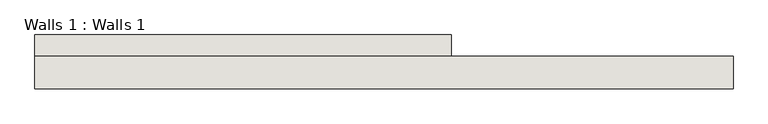
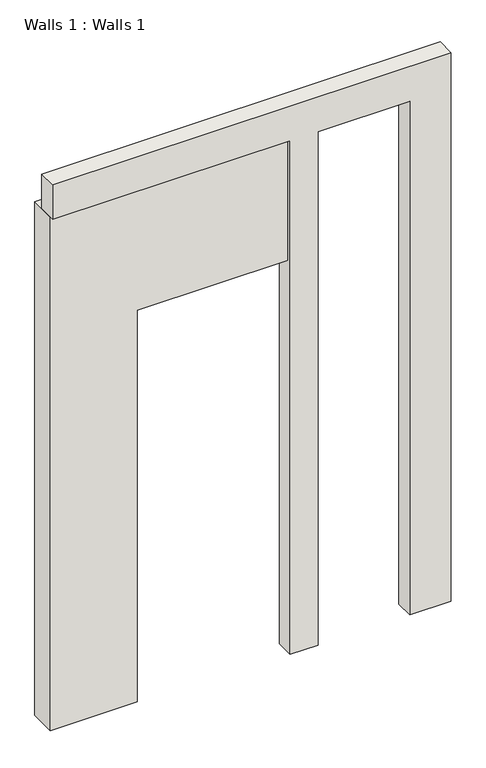
"""IFC4 building model written with IfcOpenShell, lengths in millimetres: wall geometry, Walls 1 : Walls 1."""

from ifc_helpers import new_model, si_unit, frame, origin, place, context, project, spatial, polyline, outline, extrude, source, transform, mapped, element, save


def walls_1_walls_1_01443282(model_context):
    return source(origin(), model_context, "Body", "SweptSolid", [
        extrude(outline(polyline([(0.0, -6444.1183714), (0.0, -5002.4940631), (6858.0, -5002.4940631), (6858.0, -2507.1183714), (8991.6, -2507.1183714), (8991.6, -6444.1183714), (0.0, -6444.1183714)])), frame((0.0, -461.4136201, 0.0), z_axis=(0.0, 1.0, 0.0), x_axis=(0.0, 0.0, 1.0)), (0.0, 0.0, 1.0), 441.3036572),
        extrude(outline(polyline([(9601.2, 159.8816286), (9601.2, -6444.1183714), (8991.6, -6444.1183714), (8991.6, -2507.1183714), (0.0, -2507.1183714), (0.0, -2049.9183714), (8991.6, -2049.9183714), (8991.6, -525.9183714), (0.0, -525.9183714), (0.0, 159.8816286), (9601.2, 159.8816286)])), frame((0.0, -528.1099629, 0.0), z_axis=(0.0, 1.0, 0.0), x_axis=(0.0, 0.0, 1.0)), (0.0, 0.0, 1.0), 304.8),
    ])


if __name__ == "__main__":
    model = new_model("IFC4")
    model_context = context("Model", 3, world=origin())
    ifc_project = project(units=[si_unit("LENGTHUNIT", "METRE", prefix="MILLI")], contexts=[model_context])
    site = spatial("IfcSite", under=ifc_project)
    building = spatial("IfcBuilding", under=site)
    placement = place(None, origin())
    walls_1_walls_1_shape = walls_1_walls_1_01443282(model_context)
    element("IfcWall", 1, ObjectType="Walls 1 : Walls 1", at=placement, inside=building, context=model_context, shape_type="MappedRepresentation", body=[
        mapped(walls_1_walls_1_shape, transform((0.0, 0.0, 0.0), x_axis=(1.0, 0.0, 0.0), y_axis=(0.0, 1.0, 0.0), z_axis=(0.0, 0.0, 1.0))),
    ])
    save(model, "model.ifc")

# Revit data of these elements
# Element 1 (IfcWall, "Walls 1 : Walls 1")
#   Materials on its faces: "Default Wall"
# Materials
#   "Default Wall": colour RGB 128 128 128, transparency 0
